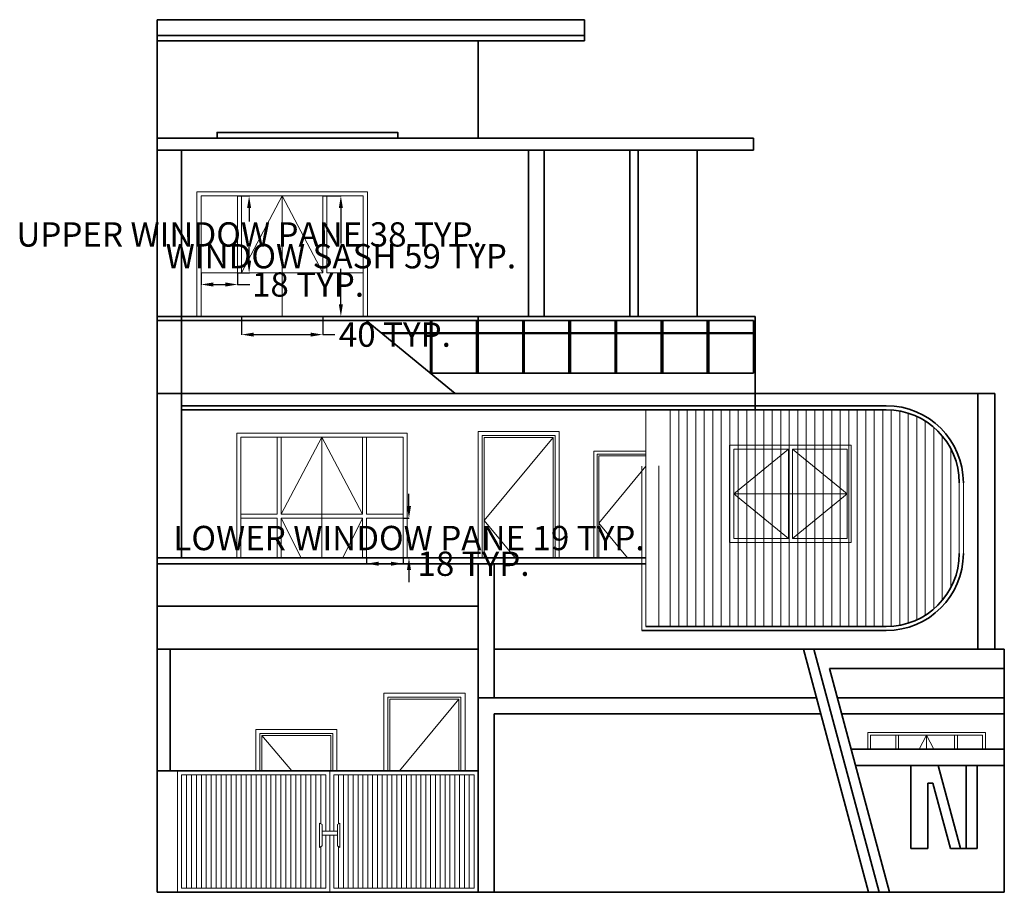
# Model space of a CAD drawing. Units: inches. Extents: x -25 to 460, y 54 to 484.
import ezdxf

# ---------------------------------------------------------------- set-up
doc = ezdxf.new("R2010")
doc.units = ezdxf.units.IN
doc.header["$MEASUREMENT"] = 0
for name, color, linetype, lineweight in [('A-ANNO-DIMS', 2, 'Continuous', 18), ('A-DOOR', 3, 'Continuous', 18), ('A-ELEV', 7, 'Continuous', 35), ('A-ELEV-PATT', 8, 'Continuous', 13), ('A-GLAZ', 4, 'Continuous', 18)]:
    doc.layers.add(name, color=color, linetype=linetype, lineweight=lineweight)
doc.styles.get("Standard").update_dxf_attribs({"font": 'arial.ttf'})
doc.dimstyles.get("Standard").update_dxf_attribs({"dimtxt": 12, "dimasz": 6, "dimexe": 0.18, "dimexo": 0.0625, "dimgap": 0.09, "dimtad": 0, "dimtih": 1, "dimtoh": 1, "dimdec": 0, "dimzin": 0, "dimdsep": 46, "dimlunit": 3, "dimtxsty": 'Standard', "dimcen": 0.09, "dimadec": 0, "dimazin": 0, "dimtfac": 1, "dimtdec": 0, "dimtofl": 0, "dimtmove": 0, "dimatfit": 3, "dimfxl": 1, "dimtolj": 1, "dimtzin": 0, "dimarcsym": 0})

# ---------------------------------------------------------------- blocks, each defined once
blk = doc.blocks.new('WIN-SASH')
for p, q in [((0, 21.49), (0, 59.49)), ((20, 59.49), (0, 21.49)), ((20, 0), (20, 59.49)), ((20, 59.49), (40, 21.49)), ((40, 21.49), (40, 59.49)), ((0, 21.49), (40, 21.49))]:
    blk.add_line(p, q)
blk = doc.blocks.new('WIN-PANE-UPPER')
for p, q in [((18, 0), (18, 38)), ((0, 0), (18, 0))]:
    blk.add_line(p, q)
blk = doc.blocks.new('WIN-PANE-LOWER')
for p, q in [((0, 0), (0, 19.49)), ((0, 19.49), (18, 19.49))]:
    blk.add_line(p, q)
blk = doc.blocks.new('*D4')
at = {"layer": 'A-ANNO-DIMS', "color": 0, "lineweight": -2, "transparency": 16777216}
for p, q in [((82.02, 397.14), (87.83, 397.14)), ((87.65, 391.14), (87.65, 384.45)), ((87.65, 365.14), (87.65, 371.84)), ((82.02, 359.14), (87.83, 359.14))]:
    blk.add_line(p, q, dxfattribs=at)
at = {"layer": 'A-ANNO-DIMS', "color": 0, "transparency": 16777216}
for points in [[(86.65, 391.14), (88.65, 391.14), (87.65, 397.14)], [(86.65, 365.14), (88.65, 365.14), (87.65, 359.14)]]:
    blk.add_solid(points, dxfattribs=at)
at = {"layer": 'Defpoints', "color": 0, "transparency": 16777216}
for p in [(81.95, 397.14), (87.65, 397.14), (81.95, 359.14)]:
    blk.add_point(p, dxfattribs=at)
at = {"layer": 'A-ANNO-DIMS', "color": 0, "transparency": 16777216, "insert": (87.65, 378.14), "char_height": 12, "attachment_point": 5}
blk.add_mtext('\\A1;UPPER WINDOW PANE 38 TYP.', dxfattribs=at)
blk = doc.blocks.new('*D5')
at = {"layer": 'A-ANNO-DIMS', "color": 0, "lineweight": -2, "transparency": 16777216}
for p, q in [((63.95, 359.08), (63.95, 353.26)), ((81.95, 359.08), (81.95, 353.26)), ((69.95, 353.44), (75.95, 353.44)), ((81.95, 353.44), (87.95, 353.44))]:
    blk.add_line(p, q, dxfattribs=at)
at = {"layer": 'A-ANNO-DIMS', "color": 0, "transparency": 16777216}
for points in [[(69.95, 354.44), (69.95, 352.44), (63.95, 353.44)], [(75.95, 354.44), (75.95, 352.44), (81.95, 353.44)]]:
    blk.add_solid(points, dxfattribs=at)
at = {"layer": 'Defpoints', "color": 0, "transparency": 16777216}
for p in [(63.95, 359.14), (81.95, 359.14), (81.95, 353.44)]:
    blk.add_point(p, dxfattribs=at)
at = {"layer": 'A-ANNO-DIMS', "color": 0, "transparency": 16777216, "insert": (116.69, 353.44), "char_height": 12, "attachment_point": 5}
blk.add_mtext('\\A1;18 TYP.', dxfattribs=at)
blk = doc.blocks.new('*D6')
at = {"layer": 'A-ANNO-DIMS', "color": 0, "lineweight": -2, "transparency": 16777216}
for p, q in [((124.02, 397.14), (133.06, 397.14)), ((132.88, 391.14), (132.88, 373.7)), ((132.88, 343.65), (132.88, 361.1)), ((124.02, 337.65), (133.06, 337.65))]:
    blk.add_line(p, q, dxfattribs=at)
at = {"layer": 'A-ANNO-DIMS', "color": 0, "transparency": 16777216}
for points in [[(131.88, 391.14), (133.88, 391.14), (132.88, 397.14)], [(131.88, 343.65), (133.88, 343.65), (132.88, 337.65)]]:
    blk.add_solid(points, dxfattribs=at)
at = {"layer": 'Defpoints', "color": 0, "transparency": 16777216}
for p in [(123.95, 397.14), (132.88, 397.14), (123.95, 337.65)]:
    blk.add_point(p, dxfattribs=at)
at = {"layer": 'A-ANNO-DIMS', "color": 0, "transparency": 16777216, "insert": (132.88, 367.4), "char_height": 12, "attachment_point": 5}
blk.add_mtext('\\A1;WINDOW SASH 59 TYP.', dxfattribs=at)
blk = doc.blocks.new('*D7')
at = {"layer": 'A-ANNO-DIMS', "color": 0, "lineweight": -2, "transparency": 16777216}
for p, q in [((83.95, 337.59), (83.95, 328.55)), ((123.95, 337.59), (123.95, 328.55)), ((89.95, 328.73), (117.95, 328.73)), ((123.95, 328.73), (129.95, 328.73))]:
    blk.add_line(p, q, dxfattribs=at)
at = {"layer": 'A-ANNO-DIMS', "color": 0, "transparency": 16777216}
for points in [[(89.95, 329.73), (89.95, 327.73), (83.95, 328.73)], [(117.95, 329.73), (117.95, 327.73), (123.95, 328.73)]]:
    blk.add_solid(points, dxfattribs=at)
at = {"layer": 'Defpoints', "color": 0, "transparency": 16777216}
for p in [(83.95, 337.65), (123.95, 337.65), (123.95, 328.73)]:
    blk.add_point(p, dxfattribs=at)
at = {"layer": 'A-ANNO-DIMS', "color": 0, "transparency": 16777216, "insert": (159.49, 328.73), "char_height": 12, "attachment_point": 5}
blk.add_mtext('\\A1;40 TYP.', dxfattribs=at)
blk = doc.blocks.new('*D8')
at = {"layer": 'A-ANNO-DIMS', "color": 0, "lineweight": -2, "transparency": 16777216}
for p, q in [((166.45, 244.14), (166.45, 250.14)), ((163.59, 238.14), (166.63, 238.14)), ((163.59, 218.65), (166.63, 218.65)), ((166.45, 212.65), (166.45, 206.65))]:
    blk.add_line(p, q, dxfattribs=at)
at = {"layer": 'A-ANNO-DIMS', "color": 0, "transparency": 16777216}
for points in [[(165.45, 244.14), (167.45, 244.14), (166.45, 238.14)], [(165.45, 212.65), (167.45, 212.65), (166.45, 218.65)]]:
    blk.add_solid(points, dxfattribs=at)
at = {"layer": 'Defpoints', "color": 0, "transparency": 16777216}
for p in [(163.53, 238.14), (166.45, 238.14), (163.53, 218.65)]:
    blk.add_point(p, dxfattribs=at)
at = {"layer": 'A-ANNO-DIMS', "color": 0, "transparency": 16777216, "insert": (166.45, 228.4), "char_height": 12, "attachment_point": 5}
blk.add_mtext('\\A1;LOWER WINDOW PANE 19 TYP.', dxfattribs=at)
blk = doc.blocks.new('*D9')
at = {"layer": 'A-ANNO-DIMS', "color": 0, "lineweight": -2, "transparency": 16777216}
for p, q in [((145.53, 218.59), (145.53, 215.55)), ((163.53, 218.59), (163.53, 215.55)), ((151.53, 215.73), (157.53, 215.73)), ((163.53, 215.73), (169.53, 215.73))]:
    blk.add_line(p, q, dxfattribs=at)
at = {"layer": 'A-ANNO-DIMS', "color": 0, "transparency": 16777216}
for points in [[(151.53, 216.73), (151.53, 214.73), (145.53, 215.73)], [(157.53, 216.73), (157.53, 214.73), (163.53, 215.73)]]:
    blk.add_solid(points, dxfattribs=at)
at = {"layer": 'Defpoints', "color": 0, "transparency": 16777216}
for p in [(145.53, 218.65), (163.53, 218.65), (163.53, 215.73)]:
    blk.add_point(p, dxfattribs=at)
at = {"layer": 'A-ANNO-DIMS', "color": 0, "transparency": 16777216, "insert": (198.26, 215.73), "char_height": 12, "attachment_point": 5}
blk.add_mtext('\\A1;18 TYP.', dxfattribs=at)

msp = doc.modelspace()

# ---------------------------------------------------------------- linework, layer by layer
at = {"layer": 'A-DOOR'}
for p, q in [((200.53, 218.65), (200.53, 281)), ((237.53, 278), (203.53, 237)), ((283.29, 263.81), (260.05, 235.79)), ((203.53, 237), (218.75, 218.65)), ((260.05, 235.79), (274.26, 218.65)), ((191.08, 148.92), (161.83, 113.65)), ((52.29, 53.65), (52.29, 113.65)), ((54.29, 55.65), (54.29, 111.65)), ((54.29, 111.65), (125.41, 111.65)), ((56.74, 55.65), (56.74, 111.65)), ((59.19, 55.65), (59.19, 111.65)), ((61.64, 55.65), (61.64, 111.65)), ((64.1, 55.65), (64.1, 111.65)), ((66.55, 55.65), (66.55, 111.65)), ((69, 55.65), (69, 111.65)), ((71.45, 55.65), (71.45, 111.65)), ((73.91, 55.65), (73.91, 111.65)), ((76.36, 55.65), (76.36, 111.65)), ((78.81, 55.65), (78.81, 111.65)), ((81.26, 55.65), (81.26, 111.65)), ((83.72, 55.65), (83.72, 111.65)), ((86.17, 55.65), (86.17, 111.65)), ((88.62, 55.65), (88.62, 111.65)), ((91.07, 55.65), (91.07, 111.65)), ((93.53, 55.65), (93.53, 111.65)), ((95.98, 55.65), (95.98, 111.65)), ((98.43, 55.65), (98.43, 111.65)), ((100.88, 55.65), (100.88, 111.65)), ((103.34, 55.65), (103.34, 111.65)), ((105.79, 55.65), (105.79, 111.65)), ((108.24, 55.65), (108.24, 111.65)), ((110.69, 55.65), (110.69, 111.65)), ((113.15, 55.65), (113.15, 111.65)), ((115.6, 55.65), (115.6, 111.65)), ((118.05, 55.65), (118.05, 111.65)), ((120.51, 55.65), (120.51, 111.65)), ((122.96, 87.51), (122.96, 111.65)), ((125.41, 83.82), (125.41, 111.65)), ((125.41, 83.82), (125.41, 111.65)), ((127.41, 83.82), (127.41, 113.65)), ((129.41, 111.65), (198.53, 111.65)), ((129.41, 83.82), (129.41, 111.65)), ((129.41, 83.82), (129.41, 111.65)), ((131.79, 87.47), (131.79, 111.65)), ((134.18, 55.65), (134.18, 111.65)), ((136.56, 55.65), (136.56, 111.65)), ((138.94, 55.65), (138.94, 111.65)), ((141.33, 55.65), (141.33, 111.65)), ((143.71, 55.65), (143.71, 111.65)), ((146.1, 55.65), (146.1, 111.65)), ((148.48, 55.65), (148.48, 111.65)), ((150.86, 55.65), (150.86, 111.65)), ((153.25, 55.65), (153.25, 111.65)), ((155.63, 55.65), (155.63, 111.65)), ((158.01, 55.65), (158.01, 111.65)), ((160.4, 55.65), (160.4, 111.65)), ((162.78, 55.65), (162.78, 111.65)), ((165.16, 55.65), (165.16, 111.65)), ((167.55, 55.65), (167.55, 111.65)), ((169.93, 55.65), (169.93, 111.65)), ((172.32, 55.65), (172.32, 111.65)), ((174.7, 55.65), (174.7, 111.65)), ((177.08, 55.65), (177.08, 111.65)), ((179.47, 55.65), (179.47, 111.65)), ((181.85, 55.65), (181.85, 111.65)), ((184.23, 55.65), (184.23, 111.65)), ((186.62, 55.65), (186.62, 111.65)), ((189, 55.65), (189, 111.65)), ((191.38, 55.65), (191.38, 111.65)), ((193.77, 55.65), (193.77, 111.65)), ((196.15, 55.65), (196.15, 111.65)), ((198.53, 55.65), (198.53, 111.65)), ((123.67, 87.09), (122.41, 87.83)), ((122.41, 87.83), (122.41, 75.81)), ((131.15, 87.09), (132.41, 87.83)), ((132.41, 87.83), (132.41, 75.81)), ((123.67, 81.82), (123.67, 87.09)), ((123.67, 83.82), (131.15, 83.82)), ((125.4, 83.82), (125.4, 86.9)), ((131.15, 81.82), (131.15, 87.09)), ((123.67, 81.82), (123.67, 76.56)), ((123.67, 81.82), (131.15, 81.82)), ((125.4, 81.64), (125.4, 81.82)), ((125.4, 81.64), (125.4, 76.37)), ((125.41, 55.65), (125.41, 81.82)), ((125.41, 55.65), (125.41, 81.82)), ((127.41, 53.65), (127.41, 81.82)), ((129.41, 55.65), (129.41, 81.82)), ((129.41, 55.65), (129.41, 81.82)), ((131.15, 81.82), (131.15, 76.56)), ((123.67, 76.56), (122.41, 75.81)), ((122.96, 55.65), (122.96, 76.14)), ((131.15, 76.56), (132.41, 75.81)), ((131.79, 55.65), (131.79, 76.18)), ((125.41, 55.65), (54.29, 55.65)), ((198.53, 55.65), (129.41, 55.65))]:
    msp.add_line(p, q, dxfattribs=at)
for points in [[(200.53, 218.65), (200.53, 281), (240.53, 281), (240.53, 218.65)], [(202.53, 218.65), (202.53, 279), (238.53, 279), (238.53, 218.65)], [(203.53, 218.65), (203.53, 278), (237.53, 278), (237.53, 218.65)], [(257.63, 218.65), (257.63, 271.31), (283.29, 271.31)], [(259.25, 218.65), (259.25, 269.69), (283.29, 269.69)], [(260.05, 218.65), (260.05, 268.88), (283.29, 268.88)], [(154.08, 113.65), (154.08, 151.92), (194.08, 151.92), (194.08, 113.65)], [(156.08, 113.65), (156.08, 149.92), (192.08, 149.92), (192.08, 113.65)], [(157.08, 113.65), (157.08, 148.92), (191.08, 148.92), (191.08, 113.65)]]:
    msp.add_lwpolyline(points, dxfattribs=at)
at = {"layer": 'A-ELEV'}
for p, q in [((42.29, 53.65), (42.29, 484.06)), ((42.29, 484.06), (252.98, 484.06)), ((252.98, 484.06), (252.98, 473.65)), ((42.29, 476.27), (252.98, 476.27)), ((42.29, 473.65), (252.98, 473.65)), ((200.53, 425.65), (200.53, 473.65)), ((42.29, 425.65), (336.29, 425.65)), ((336.29, 425.65), (336.29, 419.65)), ((42.29, 419.65), (336.29, 419.65)), ((54.29, 218.65), (54.29, 419.65)), ((225.43, 337.65), (225.43, 419.65)), ((233.06, 337.65), (233.06, 419.65)), ((275.26, 337.65), (275.26, 419.65)), ((279.52, 337.65), (279.52, 419.65)), ((308.58, 337.65), (308.58, 419.65)), ((42.29, 337.65), (336.29, 337.65)), ((42.29, 335.65), (336.29, 335.65)), ((145.39, 335.65), (189.29, 299.65)), ((176.99, 309.73), (176.99, 335.65)), ((177.8, 309.73), (177.8, 335.65)), ((199.75, 309.73), (199.75, 335.65)), ((200.53, 335.65), (200.53, 337.65)), ((200.55, 309.73), (200.55, 335.65)), ((222.51, 309.73), (222.51, 335.65)), ((223.31, 309.73), (223.31, 335.65)), ((245.26, 309.73), (245.26, 335.65)), ((246.06, 309.73), (246.06, 335.65)), ((268.02, 309.73), (268.02, 335.65)), ((268.82, 309.73), (268.82, 335.65)), ((290.77, 309.73), (290.77, 335.65)), ((291.58, 309.73), (291.58, 335.65)), ((313.53, 309.73), (313.53, 335.65)), ((314.33, 309.73), (314.33, 335.65)), ((336.29, 337.65), (337.09, 337.65)), ((336.29, 309.73), (336.29, 335.65)), ((337.09, 337.65), (337.09, 335.65)), ((337.09, 291.65), (337.09, 335.65)), ((152.85, 329.53), (336.29, 329.53)), ((153.23, 329.22), (336.29, 329.22)), ((176.99, 309.73), (336.29, 309.73)), ((42.29, 299.65), (337.09, 299.65)), ((337.09, 299.65), (455.28, 299.65)), ((446.85, 299.65), (446.85, 173.65)), ((455.28, 299.65), (455.28, 173.65)), ((54.29, 293.65), (336.29, 293.65)), ((54.29, 291.65), (336.29, 291.65)), ((283.29, 293.65), (401.74, 293.65)), ((283.29, 291.65), (401.74, 291.65)), ((42.29, 218.65), (283.29, 218.65)), ((42.29, 215.65), (283.29, 215.65)), ((200.53, 111.65), (200.53, 215.65)), ((208.53, 149.65), (208.53, 215.65)), ((42.29, 194.82), (200.53, 194.82)), ((401.74, 184.76), (283.29, 184.76)), ((401.74, 182.76), (281.29, 182.76)), ((42.29, 173.65), (200.53, 173.65)), ((48.78, 113.65), (48.78, 173.65)), ((208.53, 173.65), (459.93, 173.65)), ((360.88, 173.65), (393.03, 53.65)), ((366.05, 173.65), (398.21, 53.65)), ((459.93, 173.65), (459.93, 149.65)), ((373.78, 164.11), (403.38, 53.65)), ((373.78, 164.11), (459.93, 164.11)), ((200.53, 149.65), (367.31, 149.65)), ((377.66, 149.65), (459.93, 149.65)), ((459.93, 149.65), (459.93, 53.65)), ((208.53, 53.65), (208.53, 141.65)), ((208.53, 141.65), (369.45, 141.65)), ((379.8, 141.65), (459.93, 141.65)), ((42.29, 113.65), (200.53, 113.65)), ((200.53, 53.65), (200.53, 111.65)), ((413.9, 75.19), (413.9, 116.13)), ((438.28, 75.19), (427.31, 116.13)), ((441.16, 116.13), (441.16, 75.19)), ((446.56, 116.13), (446.56, 75.19)), ((424.7, 107.52), (422.18, 107.52)), ((422.18, 107.52), (422.18, 75.19)), ((433.37, 75.19), (424.7, 107.52)), ((422.18, 75.19), (413.9, 75.19)), ((446.56, 75.19), (433.37, 75.19)), ((42.29, 53.65), (459.93, 53.65)), ((200.53, 53.65), (54.29, 53.65))]:
    msp.add_line(p, q, dxfattribs=at)
msp.add_lwpolyline([(71.87, 425.65), (160.96, 425.65), (160.96, 428.43), (71.87, 428.43)], close=True, dxfattribs=at)
msp.add_lwpolyline([(384.44, 124.33), (459.93, 124.33), (459.93, 116.13), (386.64, 116.13)], dxfattribs=at)
for centre, radius, start, end in [((401.74, 255.65), 38, 0, 90), ((401.74, 255.65), 36, 0, 90), ((401.74, 220.76), 36, 270, 0), ((401.74, 220.76), 38, 270, 0)]:
    msp.add_arc(centre, radius, start, end, dxfattribs=at)
at = {"layer": 'A-ELEV-PATT'}
for p, q in [((283.29, 263.81), (283.29, 291.65)), ((295.29, 184.76), (295.29, 291.65)), ((299.48, 184.76), (299.48, 291.65)), ((303.67, 184.76), (303.67, 291.65)), ((307.86, 184.76), (307.86, 291.65)), ((312.05, 184.76), (312.05, 291.65)), ((316.24, 184.76), (316.24, 291.65)), ((320.43, 184.76), (320.43, 291.65)), ((324.62, 184.76), (324.62, 291.65)), ((328.81, 184.76), (328.81, 291.65)), ((333, 184.76), (333, 291.65)), ((337.19, 184.76), (337.19, 291.65)), ((341.38, 184.76), (341.38, 291.65)), ((345.57, 184.76), (345.57, 291.65)), ((349.76, 184.76), (349.76, 291.65)), ((353.95, 184.76), (353.95, 291.65)), ((358.14, 184.76), (358.14, 291.65)), ((362.33, 184.76), (362.33, 291.65)), ((366.52, 184.76), (366.52, 291.65)), ((370.71, 184.76), (370.71, 291.65)), ((374.9, 184.76), (374.9, 291.65)), ((379.09, 184.76), (379.09, 291.65)), ((383.28, 184.76), (383.28, 291.65)), ((387.47, 184.76), (387.47, 291.65)), ((391.66, 184.76), (391.66, 291.65)), ((395.85, 184.76), (395.85, 291.65)), ((400.04, 184.76), (400.04, 291.65)), ((404.23, 184.76), (404.23, 291.65)), ((408.42, 185.39), (408.42, 291.03)), ((412.6, 186.44), (412.6, 289.97)), ((416.79, 188.06), (416.79, 288.35)), ((420.98, 190.34), (420.98, 286.08)), ((425.17, 193.43), (425.17, 282.98)), ((429.36, 197.67), (429.36, 278.74)), ((433.55, 203.91), (433.55, 272.51)), ((281.29, 263.81), (281.29, 182.76)), ((283.29, 263.81), (283.29, 184.76)), ((289.56, 184.76), (289.56, 263.94)), ((437.74, 255.65), (437.74, 220.76)), ((437.74, 220.76), (437.74, 255.65)), ((439.74, 220.76), (439.74, 255.65))]:
    msp.add_line(p, q, dxfattribs=at)
at = {"layer": 'A-GLAZ'}
for p, q in [((324.52, 226.21), (324.52, 274.21)), ((324.52, 274.21), (360.52, 274.21)), ((326.52, 228.21), (326.52, 272.21)), ((326.52, 272.21), (353.52, 272.21)), ((353.52, 272.21), (326.52, 250.21)), ((353.52, 228.21), (353.52, 272.21)), ((355.52, 228.21), (355.52, 272.21)), ((355.52, 272.21), (360.52, 272.21)), ((355.52, 272.21), (382.52, 250.21)), ((360.52, 274.21), (384.52, 274.21)), ((360.52, 272.21), (382.52, 272.21)), ((382.52, 272.21), (382.52, 228.21)), ((384.52, 274.21), (384.52, 226.21)), ((326.52, 250.21), (353.52, 228.21)), ((326.52, 250.21), (382.52, 250.21)), ((382.52, 250.21), (355.52, 228.21)), ((103.53, 218.65), (103.53, 238.14)), ((103.53, 238.14), (143.53, 238.14)), ((103.53, 238.14), (113.27, 218.65)), ((143.53, 238.14), (133.78, 218.65)), ((143.53, 218.65), (143.53, 238.14)), ((353.52, 228.21), (326.52, 228.21)), ((382.52, 228.21), (355.52, 228.21)), ((384.52, 226.21), (324.52, 226.21)), ((406.42, 124.33), (406.42, 131.16)), ((407.8, 124.33), (407.8, 131.16)), ((421.61, 131.16), (418.01, 124.33)), ((421.61, 131.16), (425.2, 124.33)), ((421.61, 124.33), (421.61, 131.16)), ((435.42, 124.33), (435.42, 131.16)), ((436.8, 124.33), (436.8, 131.16)), ((93.9, 130.95), (108.7, 113.65))]:
    msp.add_line(p, q, dxfattribs=at)
for points in [[(145.95, 337.65), (145.95, 399.14), (61.95, 399.14), (61.95, 337.65)], [(143.95, 337.65), (143.95, 397.14), (63.95, 397.14), (63.95, 337.65)], [(165.53, 218.65), (165.53, 280.14), (81.53, 280.14), (81.53, 218.65)], [(163.53, 218.65), (163.53, 278.14), (83.53, 278.14), (83.53, 218.65)], [(90.9, 113.65), (90.9, 133.95), (130.9, 133.95), (130.9, 113.65)], [(92.9, 113.65), (92.9, 131.95), (128.9, 131.95), (128.9, 113.65)], [(450.61, 124.33), (450.61, 132.54), (392.61, 132.54), (392.61, 124.33)], [(449.23, 124.33), (449.23, 131.16), (393.99, 131.16), (393.99, 124.33)], [(93.9, 113.65), (93.9, 130.95), (127.9, 130.95), (127.9, 113.65)]]:
    msp.add_lwpolyline(points, dxfattribs=at)

# ---------------------------------------------------------------- block references
for name, p in [('WIN-PANE-UPPER', (63.96, 359.14)), ('WIN-SASH', (83.96, 337.65)), ('WIN-PANE-UPPER', (83.53, 240.14)), ('WIN-SASH', (103.53, 218.65)), ('WIN-PANE-LOWER', (145.53, 218.65))]:
    msp.add_blockref(name, p, dxfattribs=at)
at = {"layer": 'A-GLAZ', "extrusion": (0, 0, -1), "zscale": -1}
for name, p in [('WIN-PANE-UPPER', (-143.95, 359.14)), ('WIN-PANE-UPPER', (-163.53, 240.14)), ('WIN-PANE-LOWER', (-101.53, 218.65))]:
    msp.add_blockref(name, p, dxfattribs=at)

# ---------------------------------------------------------------- dimensions: what is measured, and where the dimension line sits
at = {"layer": 'A-ANNO-DIMS'}
for base, p1, p2, text, picture, middle in [((87.65, 397.14), (81.95, 359.14), (81.95, 397.14), 'UPPER WINDOW PANE <> TYP.', '*D4', (87.65, 378.14)), ((132.88, 397.14), (123.95, 337.65), (123.95, 397.14), 'WINDOW SASH <> TYP.', '*D6', (132.88, 367.4)), ((166.45, 238.14), (163.53, 218.65), (163.53, 238.14), 'LOWER WINDOW PANE <> TYP.', '*D8', (166.45, 228.4))]:
    dim = msp.add_linear_dim(base=base, p1=p1, p2=p2, angle=90, text=text, dimstyle='Standard', override={"dimdec": 0, "dimlfac": 1, "dimrnd": 0, "dimzin": 0, "dimdsep": 46, "dimlunit": 2}, dxfattribs=at)
    dim.commit()
    dim.dimension.update_dxf_attribs({"geometry": picture, "text_midpoint": middle})
for base, p1, p2, picture, middle in [((81.95, 353.44), (63.95, 359.14), (81.95, 359.14), '*D5', (116.69, 353.44)), ((123.95, 328.73), (83.95, 337.65), (123.95, 337.65), '*D7', (159.49, 328.73)), ((163.53, 215.73), (145.53, 218.65), (163.53, 218.65), '*D9', (198.26, 215.73))]:
    dim = msp.add_linear_dim(base=base, p1=p1, p2=p2, text='<> TYP.', dimstyle='Standard', override={"dimdec": 0, "dimlfac": 1, "dimrnd": 0, "dimzin": 0, "dimdsep": 46, "dimlunit": 2}, dxfattribs=at)
    dim.commit()
    dim.dimension.update_dxf_attribs({"geometry": picture, "text_midpoint": middle})

doc.saveas('drawing.dxf')
